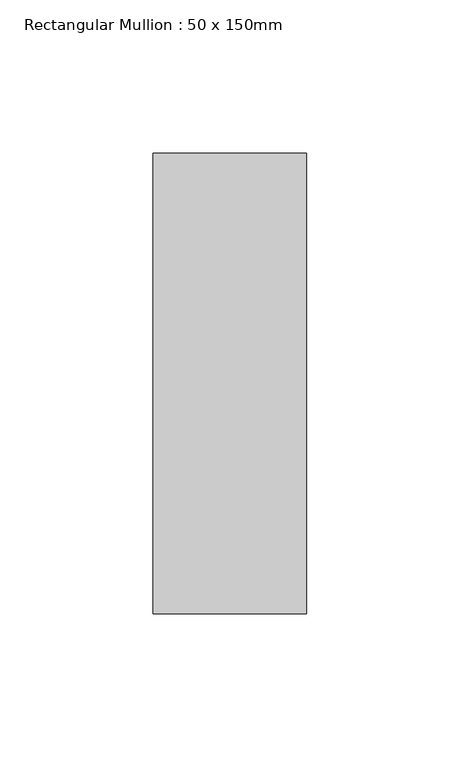
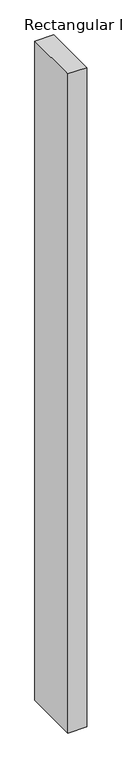
"""IFC4 building model written with IfcOpenShell, lengths in millimetres: member geometry, Rectangular Mullion : 50 x 150mm."""

from ifc_helpers import new_model, si_unit, frame, origin, place, context, project, spatial, polyline, outline, extrude, source, transform, mapped, element, save


def rectangular_mullion_50_x_150mm_8c42de37(model_context):
    return source(origin(), model_context, "Body", "SweptSolid", [
        extrude(outline(polyline([(25.0, 75.0), (25.0, -75.0), (-25.0, -75.0), (-25.0, 75.0), (25.0, 75.0)])), frame((0.0, 0.0, -1828.8), z_axis=(0.0, 0.0, 1.0), x_axis=(1.0, 0.0, 0.0)), (0.0, 0.0, 1.0), 1828.8),
    ])


if __name__ == "__main__":
    model = new_model("IFC4")
    model_context = context("Model", 3, world=origin())
    ifc_project = project(units=[si_unit("LENGTHUNIT", "METRE", prefix="MILLI")], contexts=[model_context])
    site = spatial("IfcSite", under=ifc_project)
    building = spatial("IfcBuilding", under=site)
    placement = place(None, origin())
    rectangular_mullion_50_x_150mm_shape = rectangular_mullion_50_x_150mm_8c42de37(model_context)
    element("IfcMember", 1, ObjectType="Rectangular Mullion : 50 x 150mm", at=placement, inside=building, context=model_context, shape_type="MappedRepresentation", body=[
        mapped(rectangular_mullion_50_x_150mm_shape, transform((0.0, 0.0, 0.0), x_axis=(1.0, 0.0, 0.0), y_axis=(0.0, 1.0, 0.0), z_axis=(0.0, 0.0, 1.0))),
    ])
    save(model, "model.ifc")

# Revit data of these elements
# Type "Rectangular Mullion : 50 x 150mm"
#   built-in parameter 1007304 = 0.492126 (stored number, unit not read)
#   built-in parameter 1007301 = 0.082021 (stored number, unit not read)
#   built-in parameter 1007300 = 0.082021 (stored number, unit not read)
# Element 1 (IfcMember, "Rectangular Mullion : 50 x 150mm")
#   Materials on its faces: "Aluminium"
# Materials
#   "Aluminium": class "Metal", colour RGB 247 247 247, transparency 0, Description = "Aluminium 6061", Cost = 0
